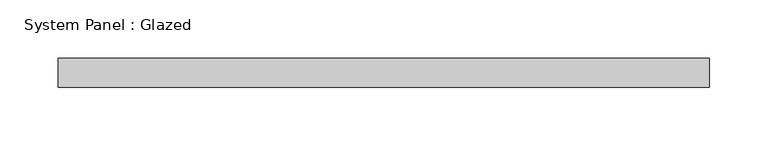
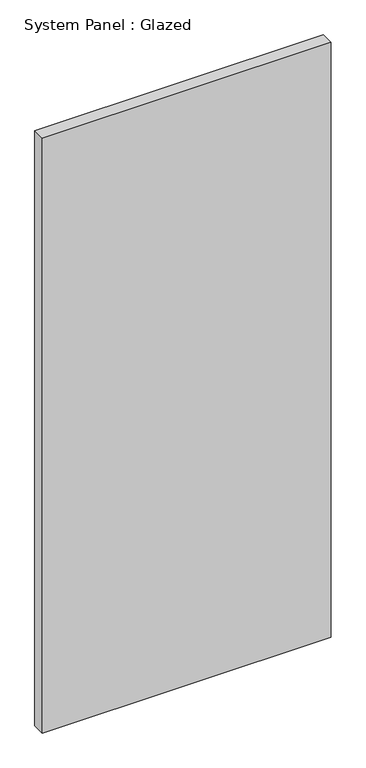
"""IFC4 building model written with IfcOpenShell, lengths in millimetres: plate geometry, System Panel : Glazed."""

from ifc_helpers import new_model, si_unit, origin, origin_with_axes, place, context, project, spatial, polyline, outline, extrude, source, transform, mapped, element, save


def system_panel_glazed_2cda0698(model_context):
    return source(origin(), model_context, "Body", "SweptSolid", [
        extrude(outline(polyline([(280.9875, 19.05), (-280.9875, 19.05), (-280.9875, 44.45), (280.9875, 44.45), (280.9875, 19.05)])), origin_with_axes(), (0.0, 0.0, 1.0), 1222.975361),
    ])


if __name__ == "__main__":
    model = new_model("IFC4")
    model_context = context("Model", 3, world=origin())
    ifc_project = project(units=[si_unit("LENGTHUNIT", "METRE", prefix="MILLI")], contexts=[model_context])
    site = spatial("IfcSite", under=ifc_project)
    building = spatial("IfcBuilding", under=site)
    placement = place(None, origin())
    system_panel_glazed_shape = system_panel_glazed_2cda0698(model_context)
    element("IfcPlate", 1, ObjectType="System Panel : Glazed", at=placement, inside=building, context=model_context, shape_type="MappedRepresentation", body=[
        mapped(system_panel_glazed_shape, transform((0.0, 0.0, 0.0), x_axis=(1.0, 0.0, 0.0), y_axis=(0.0, 1.0, 0.0), z_axis=(0.0, 0.0, 1.0))),
    ])
    save(model, "model.ifc")

# Revit data of these elements
# Type "System Panel : Glazed"
#   Construction Type Id = "GSP4R"
#   Analytic Construction = "1/8 in Pilkington single glazing"
#   Visual Light Transmittance = 0.9
#   Solar Heat Gain Coefficient = 0.86
#   Heat Transfer Coefficient (U) = 1.18115 BTU/(h·ft²·°F)
#   Define Thermal Properties by = 1
# Element 1 (IfcPlate, "System Panel : Glazed")
#   Materials on its faces: "Glass"
# Materials
#   "Glass": class "Glass", colour RGB 0 128 192, transparency 0.75, Description = "Soda Lime Glass", Cost = 0
